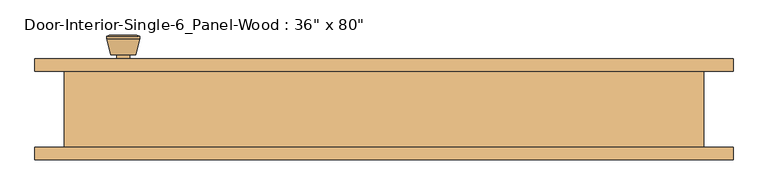
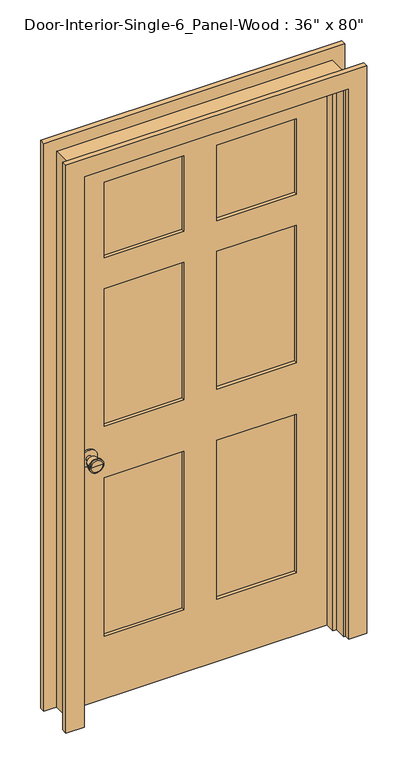
"""IFC4 building model written with IfcOpenShell, lengths in millimetres: door geometry."""

from ifc_helpers import new_model, si_unit, point, frame, frame_2d, origin, place, context, project, spatial, polyline, circle_curve, trimmed, segment, composite_curve, outline, extrude, faceted_brep, source, transform, mapped, element, save
from ifc_brep_helpers import plane_surface, cylinder_surface, revolved_surface, advanced_brep


def door_92bad2d9(model_context):
    return source(origin(), model_context, "Body", "SolidModel", [
        advanced_brep(
        [(-393.7, 13.05, 914.4), (-383.7, 13.05, 914.4), (-403.7, 13.05, 914.4), (-373.2241324, -35.95, 914.4), (-393.7, -35.95, 914.4), (-414.1758676, -35.95, 914.4), (-368.7, -34.1221319, 914.4), (-418.7, -34.1221319, 914.4), (-368.7, -30.6584537, 914.4), (-418.7, -30.6584537, 914.4), (-375.063764, -5.95, 914.4), (-412.336236, -5.95, 914.4), (-383.7, -5.95, 914.4), (-403.7, -5.95, 914.4)],
        [
            (0, 1),
            (1, 2, circle_curve(frame((-393.7, 13.05, 914.4), z_axis=(0.0, 1.0, 0.0), x_axis=(-1.0, 0.0, 0.0)), 10.0)),
            (2, 0),
            (2, 1, circle_curve(frame((-393.7, 13.05, 914.4), z_axis=(0.0, 1.0, 0.0), x_axis=(-1.0, 0.0, 0.0)), 10.0)),
            (3, 4),
            (4, 5),
            (5, 3, circle_curve(frame((-393.7, -35.95, 914.4), z_axis=(0.0, -1.0, 0.0), x_axis=(-1.0, 0.0, 0.0)), 20.4758676)),
            (3, 5, circle_curve(frame((-393.7, -35.95, 914.4), z_axis=(0.0, -1.0, 0.0), x_axis=(-1.0, 0.0, 0.0)), 20.4758676)),
            (6, 3),
            (5, 7),
            (7, 6, circle_curve(frame((-393.7, -34.1221319, 914.4), z_axis=(0.0, -1.0, 0.0), x_axis=(-1.0, 0.0, 0.0)), 25.0)),
            (6, 7, circle_curve(frame((-393.7, -34.1221319, 914.4), z_axis=(0.0, -1.0, 0.0), x_axis=(-1.0, 0.0, 0.0)), 25.0)),
            (8, 6),
            (7, 9),
            (9, 8, circle_curve(frame((-393.7, -30.6584537, 914.4), z_axis=(0.0, -1.0, 0.0), x_axis=(-1.0, 0.0, 0.0)), 25.0)),
            (8, 9, circle_curve(frame((-393.7, -30.6584537, 914.4), z_axis=(0.0, -1.0, 0.0), x_axis=(-1.0, 0.0, 0.0)), 25.0)),
            (10, 8),
            (9, 11),
            (11, 10, circle_curve(frame((-393.7, -5.95, 914.4), z_axis=(0.0, -1.0, 0.0), x_axis=(-1.0, 0.0, 0.0)), 18.636236)),
            (10, 11, circle_curve(frame((-393.7, -5.95, 914.4), z_axis=(0.0, -1.0, 0.0), x_axis=(-1.0, 0.0, 0.0)), 18.636236)),
            (12, 10),
            (11, 13),
            (13, 12, circle_curve(frame((-393.7, -5.95, 914.4), z_axis=(0.0, -1.0, 0.0), x_axis=(-1.0, 0.0, 0.0)), 10.0)),
            (12, 13, circle_curve(frame((-393.7, -5.95, 914.4), z_axis=(0.0, -1.0, 0.0), x_axis=(-1.0, 0.0, 0.0)), 10.0)),
            (1, 12),
            (13, 2),
        ],
        [
            plane_surface(frame((-393.7, 13.05, 914.4), z_axis=(0.0, 1.0, 0.0), x_axis=(-1.0, 0.0, 0.0))),
            plane_surface(frame((-393.7, -35.95, 914.4), z_axis=(0.0, -1.0, 0.0), x_axis=(-1.0, 0.0, 0.0))),
            revolved_surface(polyline([(-414.1758676, -35.95, 914.4), (-418.7, -34.1221319, 914.4)]), (-393.7, 13.05, 914.4), (0.0, 1.0, 0.0)),
            cylinder_surface(frame((-393.7, 13.05, 914.4), z_axis=(0.0, 1.0, 0.0), x_axis=(-1.0, 0.0, 0.0)), 25.0),
            revolved_surface(polyline([(-418.7, -30.6584537, 914.4), (-412.336236, -5.95, 914.4)]), (-393.7, 13.05, 914.4), (0.0, 1.0, 0.0)),
            plane_surface(frame((-393.7, -5.95, 914.4), z_axis=(0.0, 1.0, 0.0), x_axis=(-1.0, 0.0, 0.0))),
            cylinder_surface(frame((-393.7, 13.05, 914.4), z_axis=(0.0, 1.0, 0.0), x_axis=(-1.0, 0.0, 0.0)), 10.0),
        ],
        [
            (0, [[1, 2, 3]]),
            (0, [[-3, 4, -1]]),
            (1, [[5, 6, 7]]),
            (1, [[-6, -5, 8]]),
            (2, [[9, -7, 10, 11]]),
            (2, [[-10, -8, -9, 12]]),
            (3, [[13, -11, 14, 15]]),
            (3, [[-14, -12, -13, 16]]),
            (4, [[17, -15, 18, 19]]),
            (4, [[-18, -16, -17, 20]]),
            (5, [[21, -19, 22, 23]]),
            (5, [[-22, -20, -21, 24]]),
            (6, [[25, -23, 26, -2]]),
            (6, [[-26, -24, -25, -4]]),
        ],
    ),
        extrude(outline(composite_curve([segment(trimmed(circle_curve(frame_2d((914.4, -393.7)), 30.0), [point((914.4, -423.7))], [point((914.4, -363.7))], False, "CARTESIAN"), True, "CONTINUOUS"), segment(trimmed(circle_curve(frame_2d((914.4, -393.7)), 30.0), [point((914.4, -363.7))], [point((914.4, -423.7))], False, "CARTESIAN"), True, "CONTINUOUS")], self_intersect=False)), frame((0.0, 13.05, 0.0), z_axis=(0.0, 1.0, 0.0), x_axis=(0.0, 0.0, 1.0)), (0.0, 0.0, 1.0), 6.0),
        advanced_brep(
        [(-393.7, 59.975, 914.4), (-403.7, 59.975, 914.4), (-383.7, 59.975, 914.4), (-373.2241324, 108.975, 914.4), (-414.1758676, 108.975, 914.4), (-393.7, 108.975, 914.4), (-368.7, 107.1471319, 914.4), (-418.7, 107.1471319, 914.4), (-368.7, 103.6834537, 914.4), (-418.7, 103.6834537, 914.4), (-375.063764, 78.975, 914.4), (-412.336236, 78.975, 914.4), (-383.7, 78.975, 914.4), (-403.7, 78.975, 914.4)],
        [
            (0, 1),
            (1, 2, circle_curve(frame((-393.7, 59.975, 914.4), z_axis=(0.0, -1.0, 0.0), x_axis=(-1.0, 0.0, 0.0)), 10.0)),
            (2, 0),
            (2, 1, circle_curve(frame((-393.7, 59.975, 914.4), z_axis=(0.0, -1.0, 0.0), x_axis=(-1.0, 0.0, 0.0)), 10.0)),
            (3, 4, circle_curve(frame((-393.7, 108.975, 914.4), z_axis=(0.0, 1.0, 0.0), x_axis=(-1.0, 0.0, 0.0)), 20.4758676)),
            (4, 5),
            (5, 3),
            (4, 3, circle_curve(frame((-393.7, 108.975, 914.4), z_axis=(0.0, 1.0, 0.0), x_axis=(-1.0, 0.0, 0.0)), 20.4758676)),
            (6, 7, circle_curve(frame((-393.7, 107.1471319, 914.4), z_axis=(0.0, 1.0, 0.0), x_axis=(-1.0, 0.0, 0.0)), 25.0)),
            (7, 4),
            (3, 6),
            (7, 6, circle_curve(frame((-393.7, 107.1471319, 914.4), z_axis=(0.0, 1.0, 0.0), x_axis=(-1.0, 0.0, 0.0)), 25.0)),
            (8, 9, circle_curve(frame((-393.7, 103.6834537, 914.4), z_axis=(0.0, 1.0, 0.0), x_axis=(-1.0, 0.0, 0.0)), 25.0)),
            (9, 7),
            (6, 8),
            (9, 8, circle_curve(frame((-393.7, 103.6834537, 914.4), z_axis=(0.0, 1.0, 0.0), x_axis=(-1.0, 0.0, 0.0)), 25.0)),
            (10, 11, circle_curve(frame((-393.7, 78.975, 914.4), z_axis=(0.0, 1.0, 0.0), x_axis=(-1.0, 0.0, 0.0)), 18.636236)),
            (11, 9),
            (8, 10),
            (11, 10, circle_curve(frame((-393.7, 78.975, 914.4), z_axis=(0.0, 1.0, 0.0), x_axis=(-1.0, 0.0, 0.0)), 18.636236)),
            (12, 13, circle_curve(frame((-393.7, 78.975, 914.4), z_axis=(0.0, 1.0, 0.0), x_axis=(-1.0, 0.0, 0.0)), 10.0)),
            (13, 11),
            (10, 12),
            (13, 12, circle_curve(frame((-393.7, 78.975, 914.4), z_axis=(0.0, 1.0, 0.0), x_axis=(-1.0, 0.0, 0.0)), 10.0)),
            (1, 13),
            (12, 2),
        ],
        [
            plane_surface(frame((-393.7, 59.975, 914.4), z_axis=(0.0, -1.0, 0.0), x_axis=(-1.0, 0.0, 0.0))),
            plane_surface(frame((-393.7, 108.975, 914.4), z_axis=(0.0, 1.0, 0.0), x_axis=(-1.0, 0.0, 0.0))),
            revolved_surface(polyline([(-414.1758676, 108.975, 914.4), (-418.7, 107.1471319, 914.4)]), (-393.7, 59.975, 914.4), (0.0, -1.0, 0.0)),
            cylinder_surface(frame((-393.7, 59.975, 914.4), z_axis=(0.0, -1.0, 0.0), x_axis=(-1.0, 0.0, 0.0)), 25.0),
            revolved_surface(polyline([(-418.7, 103.6834537, 914.4), (-412.336236, 78.975, 914.4)]), (-393.7, 59.975, 914.4), (0.0, -1.0, 0.0)),
            plane_surface(frame((-393.7, 78.975, 914.4), z_axis=(0.0, -1.0, 0.0), x_axis=(-1.0, 0.0, 0.0))),
            cylinder_surface(frame((-393.7, 59.975, 914.4), z_axis=(0.0, -1.0, 0.0), x_axis=(-1.0, 0.0, 0.0)), 10.0),
        ],
        [
            (0, [[1, 2, 3]]),
            (0, [[-3, 4, -1]]),
            (1, [[5, 6, 7]]),
            (1, [[8, -7, -6]]),
            (2, [[9, 10, -5, 11]]),
            (2, [[12, -11, -8, -10]]),
            (3, [[13, 14, -9, 15]]),
            (3, [[16, -15, -12, -14]]),
            (4, [[17, 18, -13, 19]]),
            (4, [[20, -19, -16, -18]]),
            (5, [[21, 22, -17, 23]]),
            (5, [[24, -23, -20, -22]]),
            (6, [[-2, 25, -21, 26]]),
            (6, [[-4, -26, -24, -25]]),
        ],
    ),
        extrude(outline(composite_curve([segment(trimmed(circle_curve(frame_2d((914.4, -393.7)), 30.0), [point((914.4, -423.7))], [point((914.4, -363.7))], False, "CARTESIAN"), True, "CONTINUOUS"), segment(trimmed(circle_curve(frame_2d((914.4, -393.7)), 30.0), [point((914.4, -363.7))], [point((914.4, -423.7))], False, "CARTESIAN"), True, "CONTINUOUS")], self_intersect=False)), frame((0.0, 53.975, 0.0), z_axis=(0.0, 1.0, 0.0), x_axis=(0.0, 0.0, 1.0)), (0.0, 0.0, 1.0), 6.0),
        faceted_brep([(482.6, 53.975, 0.0), (482.6, -60.325, 0.0), (457.2, -60.325, 0.0), (457.2, -15.875, 0.0), (444.5, -15.875, 0.0), (444.5, 19.05, 0.0), (457.2, 19.05, 0.0), (457.2, 53.975, 0.0), (482.6, 53.975, 2057.4), (482.6, -60.325, 2057.4), (-482.6, -60.325, 2057.4), (-482.6, -60.325, 0.0), (-457.2, -60.325, 0.0), (-457.2, -60.325, 2032.0), (457.2, -60.325, 2032.0), (457.2, -15.875, 2032.0), (-457.2, -15.875, 2032.0), (-457.2, -15.875, 0.0), (-444.5, -15.875, 0.0), (-444.5, -15.875, 2019.3), (444.5, -15.875, 2019.3), (444.5, 19.05, 2019.3), (-444.5, 19.05, 2019.3), (-444.5, 19.05, 0.0), (-457.2, 19.05, 0.0), (-457.2, 19.05, 2032.0), (457.2, 19.05, 2032.0), (457.2, 53.975, 2032.0), (-457.2, 53.975, 2032.0), (-457.2, 53.975, 0.0), (-482.6, 53.975, 0.0), (-482.6, 53.975, 2057.4)], [[[0, 1, 2, 3, 4, 5, 6, 7]], [[1, 0, 8, 9]], [[2, 1, 9, 10, 11, 12, 13, 14]], [[3, 2, 14, 15]], [[4, 3, 15, 16, 17, 18, 19, 20]], [[5, 4, 20, 21]], [[6, 5, 21, 22, 23, 24, 25, 26]], [[7, 6, 26, 27]], [[0, 7, 27, 28, 29, 30, 31, 8]], [[9, 8, 31, 10]], [[15, 14, 13, 16]], [[21, 20, 19, 22]], [[27, 26, 25, 28]], [[30, 29, 24, 23, 18, 17, 12, 11]], [[10, 31, 30, 11]], [[16, 13, 12, 17]], [[22, 19, 18, 23]], [[28, 25, 24, 29]]]),
        extrude(outline(polyline([(2032.0, -457.2), (0.0, -457.2), (0.0, 457.2), (2032.0, 457.2), (2032.0, -457.2)]), holes=[polyline([(1912.9375, 57.15), (1912.9375, 336.55), (1633.5375, 336.55), (1633.5375, 57.15), (1912.9375, 57.15)]), polyline([(1519.2375, 336.55), (1009.65, 336.55), (1009.65, 57.15), (1519.2375, 57.15), (1519.2375, 336.55)]), polyline([(1009.65, -57.15), (1009.65, -336.55), (1519.2375, -336.55), (1519.2375, -57.15), (1009.65, -57.15)]), polyline([(1633.5375, -336.55), (1912.9375, -336.55), (1912.9375, -57.15), (1633.5375, -57.15), (1633.5375, -336.55)]), polyline([(819.15, 57.15), (819.15, 336.55), (231.775, 336.55), (231.775, 57.15), (819.15, 57.15)]), polyline([(231.775, -57.15), (231.775, -336.55), (819.15, -336.55), (819.15, -57.15), (231.775, -57.15)])]), frame((0.0, 19.05, 0.0), z_axis=(0.0, 1.0, 0.0), x_axis=(0.0, 0.0, 1.0)), (0.0, 0.0, 1.0), 34.925),
        extrude(outline(polyline([(336.55, 30.6916667), (57.15, 30.6916667), (57.15, 42.3333333), (336.55, 42.3333333), (336.55, 30.6916667)])), frame((0.0, 0.0, 1633.5375), z_axis=(0.0, 0.0, 1.0), x_axis=(1.0, 0.0, 0.0)), (0.0, 0.0, 1.0), 279.4),
        extrude(outline(polyline([(336.55, 30.6916667), (57.15, 30.6916667), (57.15, 42.3333333), (336.55, 42.3333333), (336.55, 30.6916667)])), frame((0.0, 0.0, 1009.65), z_axis=(0.0, 0.0, 1.0), x_axis=(1.0, 0.0, 0.0)), (0.0, 0.0, 1.0), 509.5875),
        extrude(outline(polyline([(-57.15, 30.6916667), (-336.55, 30.6916667), (-336.55, 42.3333333), (-57.15, 42.3333333), (-57.15, 30.6916667)])), frame((0.0, 0.0, 1009.65), z_axis=(0.0, 0.0, 1.0), x_axis=(1.0, 0.0, 0.0)), (0.0, 0.0, 1.0), 509.5875),
        extrude(outline(polyline([(-57.15, 30.6916667), (-336.55, 30.6916667), (-336.55, 42.3333333), (-57.15, 42.3333333), (-57.15, 30.6916667)])), frame((0.0, 0.0, 1633.5375), z_axis=(0.0, 0.0, 1.0), x_axis=(1.0, 0.0, 0.0)), (0.0, 0.0, 1.0), 279.4),
        extrude(outline(polyline([(336.55, 30.6916667), (57.15, 30.6916667), (57.15, 42.3333333), (336.55, 42.3333333), (336.55, 30.6916667)])), frame((0.0, 0.0, 231.775), z_axis=(0.0, 0.0, 1.0), x_axis=(1.0, 0.0, 0.0)), (0.0, 0.0, 1.0), 587.375),
        extrude(outline(polyline([(-57.15, 30.6916667), (-336.55, 30.6916667), (-336.55, 42.3333333), (-57.15, 42.3333333), (-57.15, 30.6916667)])), frame((0.0, 0.0, 231.775), z_axis=(0.0, 0.0, 1.0), x_axis=(1.0, 0.0, 0.0)), (0.0, 0.0, 1.0), 587.375),
        extrude(outline(polyline([(0.0, 463.55), (0.0, 527.05), (2101.85, 527.05), (2101.85, -527.05), (0.0, -527.05), (0.0, -463.55), (2038.35, -463.55), (2038.35, 463.55), (0.0, 463.55)])), frame((0.0, 53.975, 0.0), z_axis=(0.0, 1.0, 0.0), x_axis=(0.0, 0.0, 1.0)), (0.0, 0.0, 1.0), 19.05),
        extrude(outline(polyline([(0.0, 463.55), (0.0, 527.05), (2101.85, 527.05), (2101.85, -527.05), (0.0, -527.05), (0.0, -463.55), (2038.35, -463.55), (2038.35, 463.55), (0.0, 463.55)])), frame((0.0, -79.375, 0.0), z_axis=(0.0, 1.0, 0.0), x_axis=(0.0, 0.0, 1.0)), (0.0, 0.0, 1.0), 19.05),
    ])


if __name__ == "__main__":
    model = new_model("IFC4")
    model_context = context("Model", 3, world=origin())
    ifc_project = project(units=[si_unit("LENGTHUNIT", "METRE", prefix="MILLI")], contexts=[model_context])
    site = spatial("IfcSite", under=ifc_project)
    building = spatial("IfcBuilding", under=site)
    placement = place(None, origin())
    door_shape = door_92bad2d9(model_context)
    element("IfcDoor", 1, ObjectType="Door-Interior-Single-6_Panel-Wood : 36\" x 80\"", at=placement, inside=building, context=model_context, shape_type="MappedRepresentation", body=[
        mapped(door_shape, transform((0.0, 0.0, 0.0), x_axis=(1.0, 0.0, 0.0), y_axis=(0.0, 1.0, 0.0), z_axis=(0.0, 0.0, 1.0))),
    ])
    save(model, "model.ifc")

# Revit data of these elements
# Type "Door-Interior-Single-6_Panel-Wood : 36\" x 80\""
#   Type Mark = "9"
#   Assembly Code = "C1020300"
#   Analytic Construction = "Wooden"
#   Top Rail = 0' - 4 11/16"
#   Top Panel = 0' - 11"
#   Thickness = 0' - 1 3/8"
#   Thermal Resistance (R) = 2.5876 (h·ft²·°F)/BTU
#   Swing Angle [instance default] = 90.00°
#   Stiles = 0' - 4 3/4"
#   Rough Width = 3' - 2"
#   Rough Height = 6' - 9"
#   Mullion = 0' - 4 1/2"
#   Lock Rail = 0' - 7 1/2"
#   Intermediate Rail = 0' - 4 1/2"
#   Height = 6' - 8"
#   Width = 3' - 0"
#   Heat Transfer Coefficient (U) = 0.3865 BTU/(h·ft²·°F)
#   Bottom Rail = 0' - 9 1/8"
#   Trim Material = Cherry
#   Panel Material = Cherry
#   Frame Material = Cherry
#   Door Handle Material = Aluminum
#   Visual Light Transmittance = 0
#   Solar Heat Gain Coefficient = 0
#   Wall Closure = (empty or 0)
#   Function = (empty or 0)
# Element 1 (IfcDoor, "Door-Interior-Single-6_Panel-Wood : 36\" x 80\"")
#   Materials on its faces: "Cherry", "Aluminum"
# Materials
#   "Cherry": class "Wood", colour RGB 226 177 128, transparency 0, Description = "Prunus Serotina", Cost = 0
#   "Aluminum": class "Metal", colour RGB 247 247 247, transparency 0, Description = "Aluminum 6061", Cost = 0
